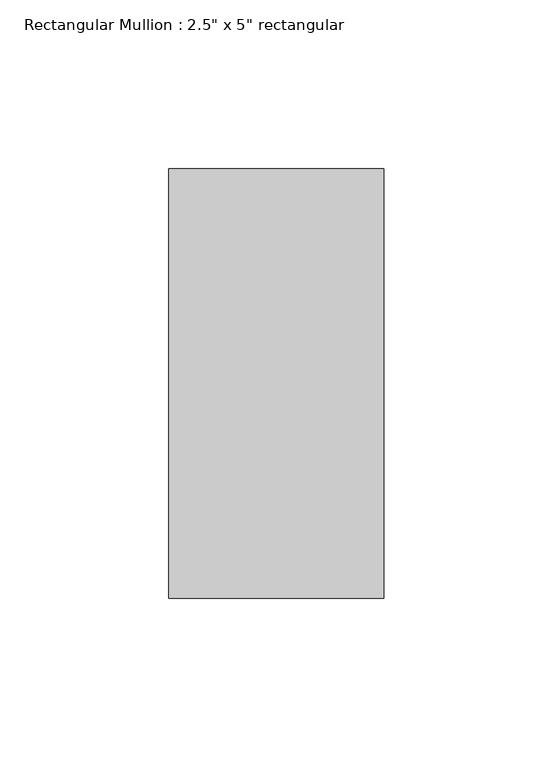
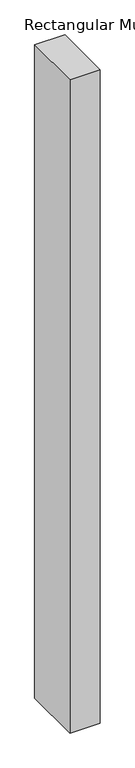
"""IFC4 building model written with IfcOpenShell, lengths in millimetres: member geometry."""

from ifc_helpers import new_model, si_unit, frame, origin, place, context, project, spatial, polyline, outline, extrude, source, transform, mapped, element, save


def member_6ca94d07(model_context):
    return source(origin(), model_context, "Body", "SweptSolid", [
        extrude(outline(polyline([(31.75, 63.5), (31.75, -63.5), (-31.75, -63.5), (-31.75, 63.5), (31.75, 63.5)])), frame((0.0, 0.0, -1442.3193903), z_axis=(0.0, 0.0, 1.0), x_axis=(1.0, 0.0, 0.0)), (0.0, 0.0, 1.0), 1442.3193903),
    ])


if __name__ == "__main__":
    model = new_model("IFC4")
    model_context = context("Model", 3, world=origin())
    ifc_project = project(units=[si_unit("LENGTHUNIT", "METRE", prefix="MILLI")], contexts=[model_context])
    site = spatial("IfcSite", under=ifc_project)
    building = spatial("IfcBuilding", under=site)
    placement = place(None, origin())
    member_shape = member_6ca94d07(model_context)
    element("IfcMember", 1, ObjectType="Rectangular Mullion : 2.5\" x 5\" rectangular", at=placement, inside=building, context=model_context, shape_type="MappedRepresentation", body=[
        mapped(member_shape, transform((0.0, 0.0, 0.0), x_axis=(1.0, 0.0, 0.0), y_axis=(0.0, 1.0, 0.0), z_axis=(0.0, 0.0, 1.0))),
    ])
    save(model, "model.ifc")

# Revit data of these elements
# Type "Rectangular Mullion : 2.5\" x 5\" rectangular"
#   built-in parameter 1007304 = 0.416667 (stored number, unit not read)
#   built-in parameter 1007301 = 0.104167 (stored number, unit not read)
#   built-in parameter 1007300 = 0.104167 (stored number, unit not read)
# Element 1 (IfcMember, "Rectangular Mullion : 2.5\" x 5\" rectangular")
#   Materials on its faces: "Aluminum"
# Materials
#   "Aluminum": class "Metal", colour RGB 247 247 247, transparency 0, Description = "Aluminum 6061", Cost = 0
